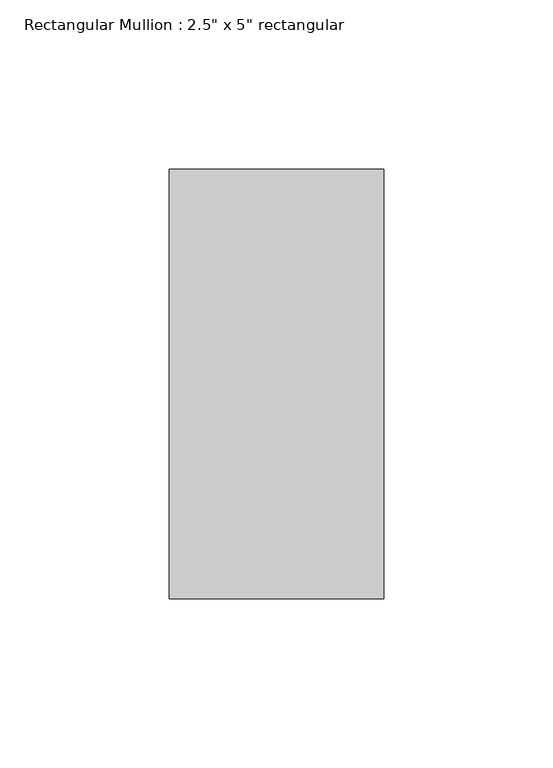
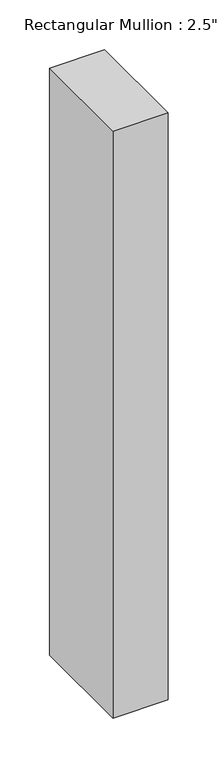
"""IFC4 building model written with IfcOpenShell, lengths in millimetres: member geometry."""

from ifc_helpers import new_model, si_unit, frame, origin, place, context, project, spatial, polyline, outline, extrude, source, transform, mapped, element, save


def member_7007ad49(model_context):
    return source(origin(), model_context, "Body", "SweptSolid", [
        extrude(outline(polyline([(0.0, 63.5), (0.0, -63.5), (-63.5, -63.5), (-63.5, 63.5), (0.0, 63.5)])), frame((0.0, 0.0, -717.55), z_axis=(0.0, 0.0, 1.0), x_axis=(1.0, 0.0, 0.0)), (0.0, 0.0, 1.0), 717.55),
    ])


if __name__ == "__main__":
    model = new_model("IFC4")
    model_context = context("Model", 3, world=origin())
    ifc_project = project(units=[si_unit("LENGTHUNIT", "METRE", prefix="MILLI")], contexts=[model_context])
    site = spatial("IfcSite", under=ifc_project)
    building = spatial("IfcBuilding", under=site)
    placement = place(None, origin())
    member_shape = member_7007ad49(model_context)
    element("IfcMember", 1, ObjectType="Rectangular Mullion : 2.5\" x 5\" rectangular", at=placement, inside=building, context=model_context, shape_type="MappedRepresentation", body=[
        mapped(member_shape, transform((0.0, 0.0, 0.0), x_axis=(1.0, 0.0, 0.0), y_axis=(0.0, 1.0, 0.0), z_axis=(0.0, 0.0, 1.0))),
    ])
    save(model, "model.ifc")

# Revit data of these elements
# Type "Rectangular Mullion : 2.5\" x 5\" rectangular"
#   built-in parameter 1007304 = 0.416667 (stored number, unit not read)
#   built-in parameter 1007301 = 0.104167 (stored number, unit not read)
#   built-in parameter 1007300 = 0.104167 (stored number, unit not read)
# Element 1 (IfcMember, "Rectangular Mullion : 2.5\" x 5\" rectangular")
#   Materials on its faces: "Aluminum"
# Materials
#   "Aluminum": class "Metal", colour RGB 247 247 247, transparency 0, Description = "Aluminum 6061", Cost = 0
